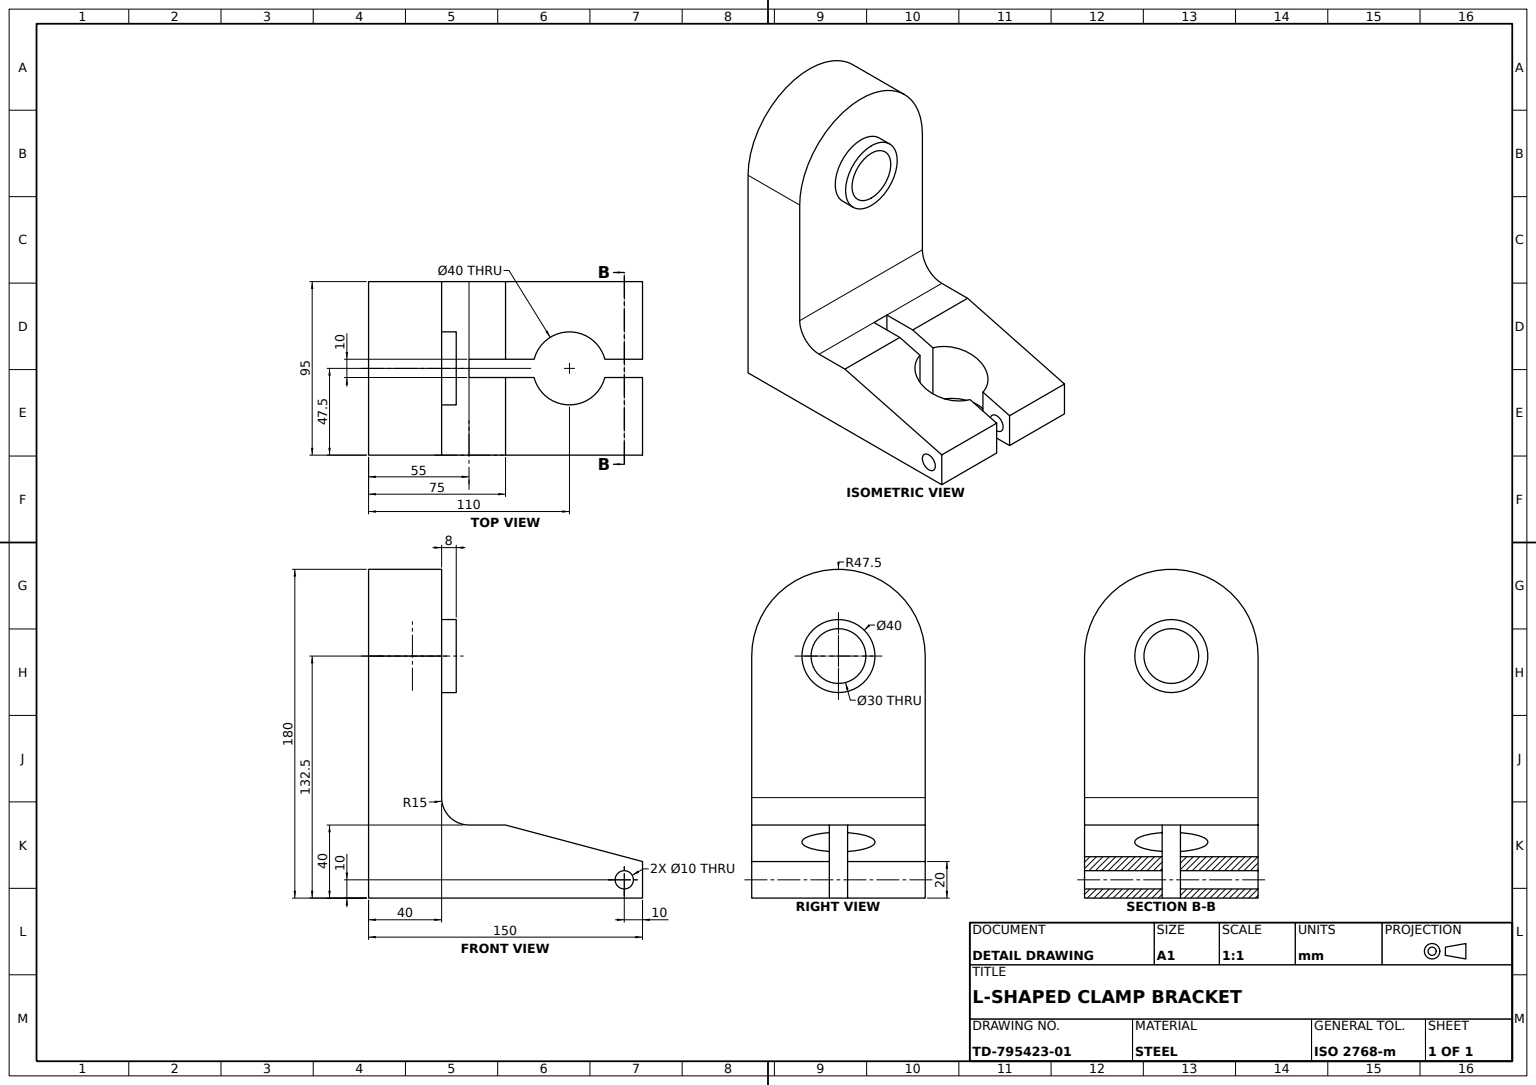
SolidWorks part; units mm, degrees
material "Plain Carbon Steel"
ref_plane "Front Plane" through (0, 0, 0) normal (0, 0, 1) x (1, 0, 0)
ref_plane "Top Plane" through (0, 0, 0) normal (0, 1, 0) x (1, 0, 0)
ref_plane "Right Plane" through (0, 0, 0) normal (1, 0, 0) x (0, 0, -1)
sketch "L-Bracket Profile Sketch" plane through (0, 0, 0) normal (0, 0, 1) x (1, 0, 0)
  line L0 (0, 0) -> (150, 0)
  line L1 (150, 0) -> (150, 20)
  line L2 (150, 20) -> (75, 40)
  line L3 (75, 40) -> (55, 40)
  line L4 (0, 0) -> (0, 132.5)
  line L5 (0, 132.5) -> (40, 132.5)
  line L6 (40, 132.5) -> (40, 55)
  arc A0 (55, 40) -> (40, 55) centre (55, 55) cw
  dimension "D7" = 15
  dimension "D1" = 132.5
  dimension "D2" = 150
  dimension "D3" = 40
  dimension "D4" = 20
  dimension "D5" = 40
  dimension "D6" = 75
extrude "L-Bracket Body" add sketch "L-Bracket Profile Sketch" along normal mid plane 95
sketch "Upright Round Top Sketch" plane through (0, 0, 0) normal (-1, 0, 0) x (0, 0, 1)
  line L0 (47.5, 132.5) -> (-47.5, 132.5) construction
  line L1 (-47.5, 132.5) -> (-47.5, 0) construction
  line L2 (-47.5, 132.5) -> (47.5, 132.5)
  arc A0 (47.5, 132.5) -> (-47.5, 132.5) centre (0, 132.5) ccw
extrude "Upright Round Top" add sketch "Upright Round Top Sketch" against normal up to surface (40 mm away) up to face at (40, 93.75, 0)
sketch "Hub Boss Ø40 Sketch" plane through (40, 0, 0) normal (1, 0, 0) x (0, 0, -1)
  circle A0 centre (0, 132.5) radius 20
  arc A3 (47.5, 132.5) -> (-47.5, 132.5) centre (0, 132.5) ccw construction
  dimension "D1" = 40
extrude "Hub Boss Ø40" add sketch "Hub Boss Ø40 Sketch" along normal blind 8
sketch "Bearing Bore Ø30 Sketch" plane through (48, 0, 0) normal (1, 0, 0) x (0, 0, -1)
  circle A0 centre (0, 132.5) radius 15
  dimension "D1" = 30
extrude "Bearing Bore Ø30" cut sketch "Bearing Bore Ø30 Sketch" against normal blind 65
sketch "Clamp Bore Ø40 Slot Sketch" plane through (0, 40, 0) normal (0, 1, 0) x (1, 0, 0)
  line L0 (150, 5) -> (150, -5)
  line L2 (129.3649, -5) -> (150, -5)
  line L3 (129.3649, 5) -> (150, 5)
  line L4 (90.6351, 5) -> (55, 5)
  line L5 (55, -47.5) -> (55, 47.5) construction
  line L6 (55, -5) -> (90.6351, -5)
  line L7 (55, 5) -> (55, -5)
  line L8 (150, -47.5) -> (150, 47.5) construction
  line L9 (110, 0) -> (116.0228, 0) construction
  arc A0 (129.3649, 5) -> (90.6351, 5) centre (110, 0) ccw
  arc A1 (90.6351, -5) -> (129.3649, -5) centre (110, 0) ccw
  dimension "D1" = 40
  dimension "D2" = 10
  dimension "D3" = 40
extrude "Clamp Bore Ø40 with Slot" cut sketch "Clamp Bore Ø40 Slot Sketch" against normal blind 65
sketch "Clamp Screw Hole Ø10 Sketch" plane through (0, 0, 47.5) normal (0, 0, 1) x (1, 0, 0)
  line L0 (0, 0) -> (150, 0) construction
  line L1 (150, 0) -> (150, 20) construction
  circle A0 centre (140, 10) radius 5
  dimension "D1" = 10
  dimension "D2" = 10
  dimension "D3" = 10
extrude "Clamp Screw Hole Ø10" cut sketch "Clamp Screw Hole Ø10 Sketch" against normal through all
